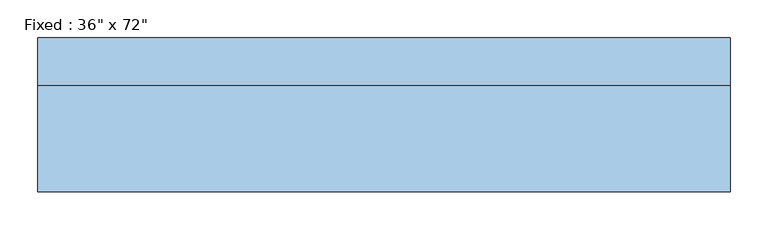
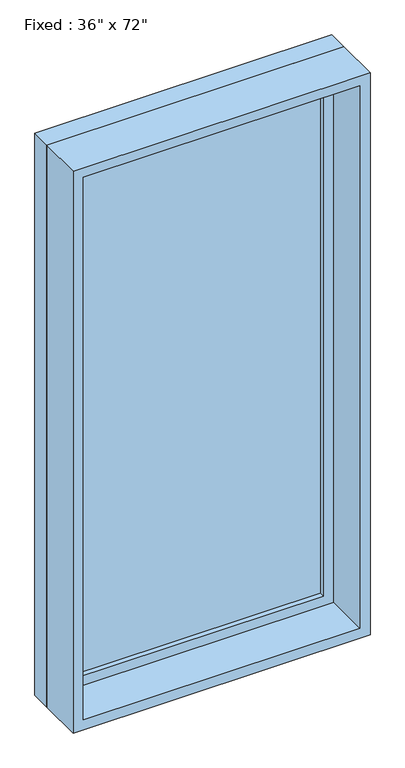
"""IFC4 building model written with IfcOpenShell, lengths in millimetres: window geometry."""

from ifc_helpers import new_model, si_unit, frame, origin, place, context, project, spatial, polyline, outline, extrude, source, transform, mapped, element, save


def window_9a779fa2(model_context):
    return source(origin(), model_context, "Body", "SweptSolid", [
        extrude(outline(polyline([(355.6, 53.975), (-431.8, 53.975), (-431.8, 66.675), (355.6, 66.675), (355.6, 53.975)])), frame((0.0, 0.0, 368.3), z_axis=(0.0, 0.0, 1.0), x_axis=(1.0, 0.0, 0.0)), (0.0, 0.0, 1.0), 1701.8),
        extrude(outline(polyline([(2114.55, -476.25), (323.85, -476.25), (323.85, 400.05), (2114.55, 400.05), (2114.55, -476.25)]), holes=[polyline([(2070.1, -431.8), (2070.1, 355.6), (368.3, 355.6), (368.3, -431.8), (2070.1, -431.8)])]), frame((0.0, 38.1, 0.0), z_axis=(0.0, 1.0, 0.0), x_axis=(0.0, 0.0, 1.0)), (0.0, 0.0, 1.0), 44.45),
        extrude(outline(polyline([(2133.6, -495.3), (304.8, -495.3), (304.8, 419.1), (2133.6, 419.1), (2133.6, -495.3)]), holes=[polyline([(2101.85, -463.55), (2101.85, 387.35), (336.55, 387.35), (336.55, -463.55), (2101.85, -463.55)])]), frame((0.0, -101.6, 0.0), z_axis=(0.0, 1.0, 0.0), x_axis=(0.0, 0.0, 1.0)), (0.0, 0.0, 1.0), 139.7),
        extrude(outline(polyline([(2133.6, 419.1), (2133.6, -495.3), (304.8, -495.3), (304.8, 419.1), (2133.6, 419.1)]), holes=[polyline([(2114.55, 400.05), (323.85, 400.05), (323.85, -476.25), (2114.55, -476.25), (2114.55, 400.05)])]), frame((0.0, 38.1, 0.0), z_axis=(0.0, 1.0, 0.0), x_axis=(0.0, 0.0, 1.0)), (0.0, 0.0, 1.0), 63.5),
    ])


if __name__ == "__main__":
    model = new_model("IFC4")
    model_context = context("Model", 3, world=origin())
    ifc_project = project(units=[si_unit("LENGTHUNIT", "METRE", prefix="MILLI")], contexts=[model_context])
    site = spatial("IfcSite", under=ifc_project)
    building = spatial("IfcBuilding", under=site)
    placement = place(None, origin())
    window_shape = window_9a779fa2(model_context)
    element("IfcWindow", 1, ObjectType="Fixed : 36\" x 72\"", at=placement, inside=building, context=model_context, shape_type="MappedRepresentation", body=[
        mapped(window_shape, transform((0.0, 0.0, 0.0), x_axis=(1.0, 0.0, 0.0), y_axis=(0.0, 1.0, 0.0), z_axis=(0.0, 0.0, 1.0))),
    ])
    save(model, "model.ifc")

# Revit data of these elements
# Type "Fixed : 36\" x 72\""
#   Type Mark = "9"
#   Assembly Code = "B2020100"
#   Height = 6' - 0"
#   Default Sill Height = 1' - 0"
#   Width = 3' - 0"
#   Window Inset = 0' - 0 3/4"
#   Glass Pane Material = Glass
#   Sash Material = Sash
#   Wall Closure = (empty or 0)
# Element 1 (IfcWindow, "Fixed : 36\" x 72\"")
#   Materials on its faces: "Sash", "Glass"
# Materials
#   "Glass": class "Glass", colour RGB 218 227 224, transparency 0.85, Description = "Soda Lime Glass", Cost = 0
#   "Sash": class "Wood", colour RGB 136 99 55, transparency 0
